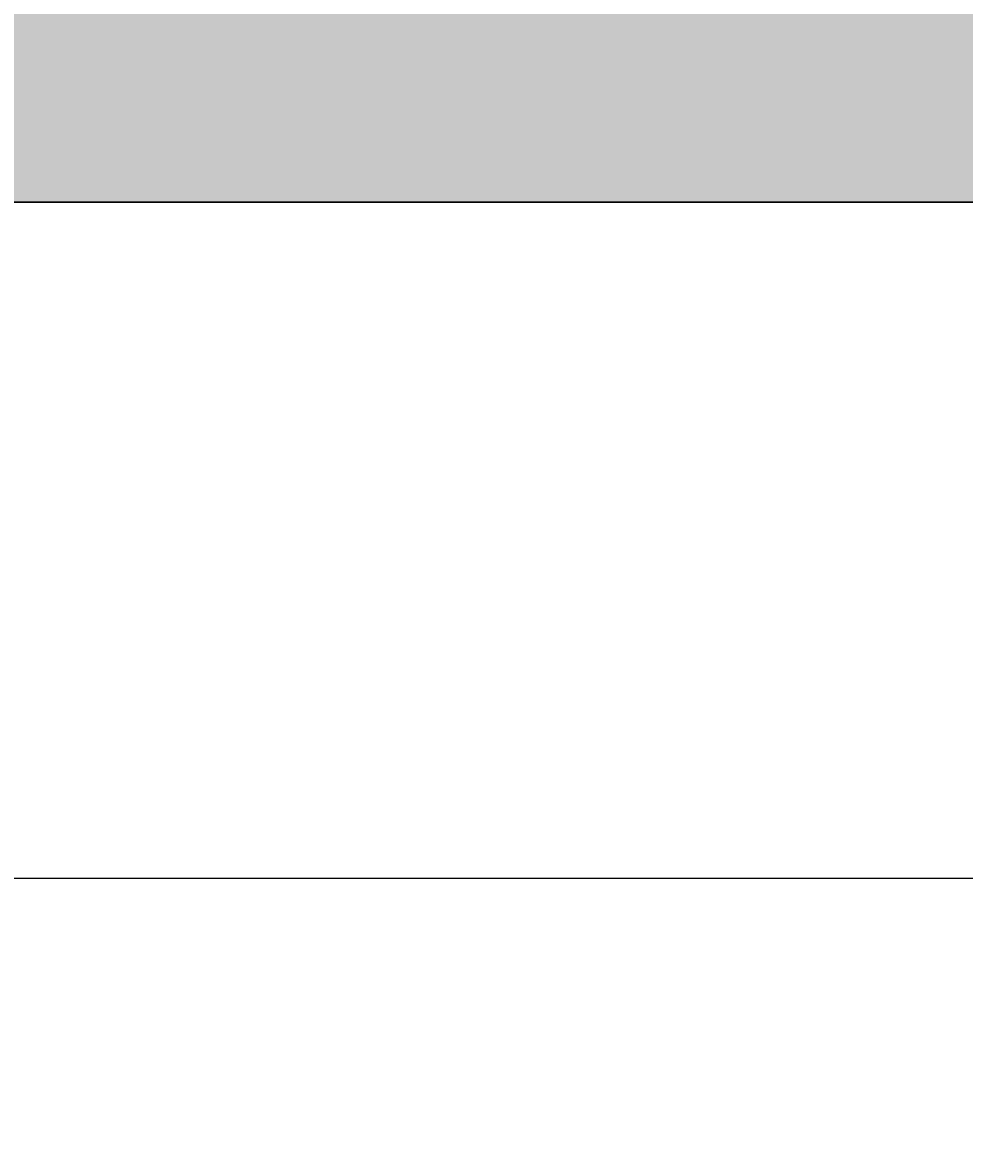
# Model space of a CAD drawing. Units: inches. Extents: x -301 to 715, y -607 to 364.
# Tile 17 of 141: x 59 to 101, y -524 to -474. Entities that reach past the tile are written whole.
import ezdxf

# ---------------------------------------------------------------- set-up
doc = ezdxf.new("R2010")
doc.units = ezdxf.units.IN
doc.header["$MEASUREMENT"] = 0
for name, color, linetype, lineweight in [('A-ANNO-DIMS', 2, 'Continuous', 18), ('A-GRND', 7, 'Continuous', 25), ('A-SECT-PATT', 8, 'Continuous', 13)]:
    doc.layers.add(name, color=color, linetype=linetype, lineweight=lineweight)
doc.styles.get("Standard").update_dxf_attribs({"font": 'arial.ttf'})
doc.dimstyles.get("Standard").update_dxf_attribs({"dimtxt": 0.18, "dimasz": 0.18, "dimexe": 0.18, "dimexo": 0.0625, "dimgap": 0.09, "dimtad": 0, "dimtih": 1, "dimtoh": 1, "dimdec": 1, "dimzin": 0, "dimdsep": 46, "dimlunit": 4, "dimtxsty": 'Standard', "dimcen": 0.09, "dimclrd": 3, "dimclre": 4, "dimclrt": 6, "dimadec": 0, "dimazin": 0, "dimtfac": 1, "dimtdec": 1, "dimtofl": 0, "dimtmove": 0, "dimatfit": 3, "dimfxl": 1, "dimtfill": 2, "dimtfillclr": 51, "dimtolj": 1, "dimtzin": 0, "dimarcsym": 0})

# ---------------------------------------------------------------- blocks, each defined once
blk = doc.blocks.new('*D176')
at = {"layer": 'A-ANNO-DIMS', "color": 4, "lineweight": -2, "transparency": 16777216}
for p, q in [((148.28, -324.477), (215.605, -324.477)), ((-15.22, -540.477), (215.605, -540.477))]:
    blk.add_line(p, q, dxfattribs=at)
at = {"layer": 'A-ANNO-DIMS', "color": 3, "lineweight": -2, "transparency": 16777216}
for p, q in [((215.425, -324.657), (215.425, -432.296)), ((215.425, -540.297), (215.425, -432.659))]:
    blk.add_line(p, q, dxfattribs=at)
at = {"layer": 'A-ANNO-DIMS', "color": 3, "transparency": 16777216}
for points in [[(215.395, -324.657), (215.455, -324.657), (215.425, -324.477)], [(215.395, -540.297), (215.455, -540.297), (215.425, -540.477)]]:
    blk.add_solid(points, dxfattribs=at)
at = {"layer": 'Defpoints', "color": 0, "transparency": 16777216}
for p in [(148.218, -324.477), (-15.282, -540.477), (215.425, -540.477)]:
    blk.add_point(p, dxfattribs=at)
at = {"layer": 'A-ANNO-DIMS', "color": 6, "transparency": 16777216, "insert": (215.425, -432.477), "char_height": 0.18, "attachment_point": 5, "bg_fill": 1, "box_fill_scale": 1.25, "bg_fill_color": 51, "bg_fill_transparency": 0}
blk.add_mtext('\\A1;18\'-0"', dxfattribs=at)
blk = doc.blocks.new('*D190')
at = {"layer": 'A-ANNO-DIMS', "color": 4, "lineweight": -2, "transparency": 16777216}
for p, q in [((129.193, -481.477), (-266.112, -481.477)), ((124.193, -511.477), (-266.112, -511.477))]:
    blk.add_line(p, q, dxfattribs=at)
at = {"layer": 'A-ANNO-DIMS', "color": 3, "lineweight": -2, "transparency": 16777216}
for p, q in [((-265.932, -481.657), (-265.932, -496.296)), ((-265.932, -511.297), (-265.932, -496.659))]:
    blk.add_line(p, q, dxfattribs=at)
at = {"layer": 'A-ANNO-DIMS', "color": 3, "transparency": 16777216}
for points in [[(-265.962, -481.657), (-265.902, -481.657), (-265.932, -481.477)], [(-265.962, -511.297), (-265.902, -511.297), (-265.932, -511.477)]]:
    blk.add_solid(points, dxfattribs=at)
at = {"layer": 'Defpoints', "color": 0, "transparency": 16777216}
for p in [(129.255, -481.477), (-265.932, -511.477), (124.255, -511.477)]:
    blk.add_point(p, dxfattribs=at)
at = {"layer": 'A-ANNO-DIMS', "color": 6, "transparency": 16777216, "insert": (-265.932, -496.477), "char_height": 0.18, "attachment_point": 5, "bg_fill": 1, "box_fill_scale": 1.25, "bg_fill_color": 51, "bg_fill_transparency": 0}
blk.add_mtext('\\A1;2\'-6"', dxfattribs=at)
blk = doc.blocks.new('*D191')
at = {"layer": 'A-ANNO-DIMS', "color": 4, "lineweight": -2, "transparency": 16777216}
for p, q in [((129.193, -481.477), (-266.112, -481.477)), ((114.193, -540.477), (-266.112, -540.477))]:
    blk.add_line(p, q, dxfattribs=at)
at = {"layer": 'A-ANNO-DIMS', "color": 3, "lineweight": -2, "transparency": 16777216}
for p, q in [((-265.932, -481.657), (-265.932, -510.797)), ((-265.932, -540.297), (-265.932, -511.158))]:
    blk.add_line(p, q, dxfattribs=at)
at = {"layer": 'A-ANNO-DIMS', "color": 3, "transparency": 16777216}
for points in [[(-265.962, -481.657), (-265.902, -481.657), (-265.932, -481.477)], [(-265.962, -540.297), (-265.902, -540.297), (-265.932, -540.477)]]:
    blk.add_solid(points, dxfattribs=at)
at = {"layer": 'Defpoints', "color": 0, "transparency": 16777216}
for p in [(129.255, -481.477), (-265.932, -540.477), (114.255, -540.477)]:
    blk.add_point(p, dxfattribs=at)
at = {"layer": 'A-ANNO-DIMS', "color": 6, "transparency": 16777216, "insert": (-265.932, -510.977), "char_height": 0.18, "attachment_point": 5, "bg_fill": 1, "box_fill_scale": 1.25, "bg_fill_color": 51, "bg_fill_transparency": 0}
blk.add_mtext('\\A1;4\'-11"', dxfattribs=at)

msp = doc.modelspace()

# ---------------------------------------------------------------- hatches: boundary and pattern name
at = {"layer": 'A-SECT-PATT'}
h = msp.add_hatch(dxfattribs=at)
h.set_pattern_fill('AR-CONC', color=256, scale=0.5)
h.set_pattern_definition([(50, (10.3213, 33.8764), (3.586301, -0.31376), [0.375, -4.125]), (355, (10.3213, 33.8764), (-0.693757, 3.76096), [0.3, -3.3]), (100.45144, (10.62, 33.8502), (2.892544, 3.4472), [0.3187, -3.50571]), (46.1842, (10.3213, 34.8764), (5.336207, -0.827596), [0.5625, -6.1875]), (96.6356, (10.766, 34.8074), (4.67331, 4.870593), [0.47805, -5.25857]), (351.1842, (10.321, 34.8764), (4.67331, 4.870593), [0.45, -4.95]), (21, (10.8213, 34.6264), (2.984535, -2.013094), [0.375, -4.125]), (326, (10.8213, 34.6264), (1.216577, 3.62575), [0.3, -3.3]), (71.45144, (11.07, 34.4586), (4.201112, 1.612656), [0.3187, -3.50571]), (37.5, (10.3213, 33.8764), (0.0607993, 1.6644693), [0, -3.26, 0, -3.35, 0, -3.3125]), (7.5, (10.3213, 33.8764), (1.3153477, 1.9720586), [0, -1.91, 0, -3.185, 0, -1.2625]), (327.5, (9.2063, 33.8764), (2.6691122, -0.1127744), [0, -1.25, 0, -3.9, 0, -5.175]), (317.5, (8.7063, 33.8764), (2.915931, 0.500525), [0, -1.625, 0, -2.59, 0, -3.675])])
h.paths.add_polyline_path([(-56.282, -535.477), (-61.282, -535.477), (-61.282, -540.477), (-15.282, -540.477), (-15.282, -535.477), (-20.282, -535.477)])
h.paths.add_polyline_path([(119.255, -535.477), (114.255, -535.477), (114.255, -540.477), (163.255, -540.477), (163.255, -535.477), (158.255, -535.477)])
h.paths.add_polyline_path([(-206.282, -471.477), (-209.282, -471.477), (-209.282, -481.477), (-206.282, -481.477), (-194.282, -481.477), (-194.282, -471.477)])
h.paths.add_polyline_path([(-41.282, -481.477), (-41.282, -471.477), (-185.282, -471.477), (-185.282, -481.477), (-180.282, -481.477)])
h.paths.add_polyline_path([(134.255, -481.477), (134.255, -471.477), (-35.282, -471.477), (-35.282, -481.477), (-30.282, -481.477)])
h.paths.add_polyline_path([(155.218, -481.477), (158.218, -481.477), (158.218, -471.477), (153.218, -471.477), (143.218, -471.477), (143.218, -481.477), (148.255, -481.477)])
h.paths.add_polyline_path([(-193.88, -356.477), (-193.904, -361.477), (143.218, -361.477), (143.218, -356.477)])

# ---------------------------------------------------------------- linework, layer by layer
at = {"layer": 'A-GRND'}
msp.add_line((-206.282, -481.477), (155.218, -481.477), dxfattribs=at)

# ---------------------------------------------------------------- dimensions: what is measured, and where the dimension line sits
at = {"layer": 'A-ANNO-DIMS'}
for base, p1, p2, picture, middle in [((215.425, -540.477), (148.218, -324.477), (-15.282, -540.477), '*D176', (215.425, -432.477)), ((-265.932, -540.477), (129.255, -481.477), (114.255, -540.477), '*D191', (-265.932, -510.977)), ((-265.932, -511.477), (129.255, -481.477), (124.255, -511.477), '*D190', (-265.932, -496.477))]:
    dim = msp.add_linear_dim(base=base, p1=p1, p2=p2, angle=90, dimstyle='Standard', override={"dimdec": 1, "dimlfac": 1, "dimrnd": 0, "dimzin": 1, "dimdsep": 46, "dimlunit": 4, "dimfrac": 2}, dxfattribs=at)
    dim.commit()
    dim.dimension.update_dxf_attribs({"geometry": picture, "text_midpoint": middle})

doc.saveas('drawing.dxf')
